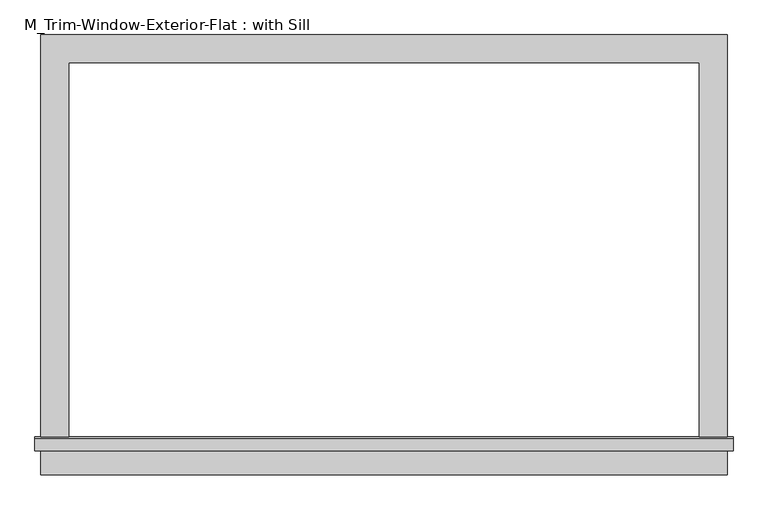
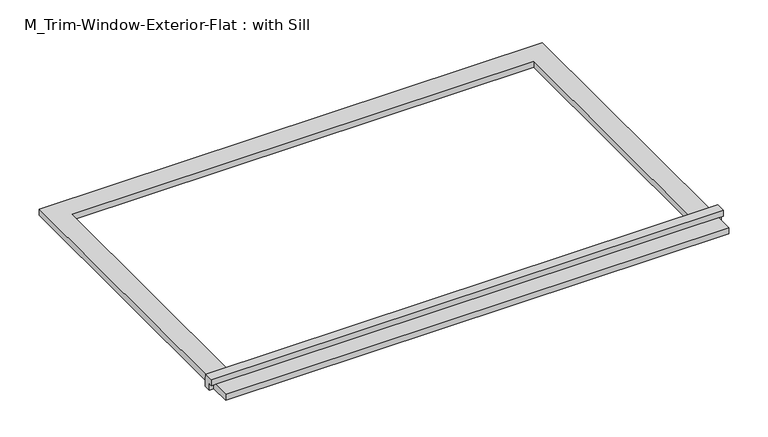
"""IFC4 building model written with IfcOpenShell, lengths in millimetres: proxy geometry, M_Trim-Window-Exterior-Flat : with Sill."""

from ifc_helpers import new_model, si_unit, frame, origin, origin_with_axes, place, context, project, spatial, polyline, outline, extrude, source, transform, mapped, element, save


def m_trim_window_exterior_flat_with_sill_2a9c44ae(model_context):
    return source(origin(), model_context, "Body", "SweptSolid", [
        extrude(outline(polyline([(733.1, -820.4323709), (733.1, -880.4323709), (-733.1, -880.4323709), (-733.1, -820.4323709), (733.1, -820.4323709)])), origin_with_axes(), (0.0, 0.0, 1.0), 19.05),
        extrude(outline(polyline([(-830.0, 38.1), (-802.4580645, 38.1), (-800.0, 19.05), (-800.0, 0.0), (-820.4323709, 0.0), (-820.4323709, 19.05), (-830.0, 19.05), (-830.0, 38.1)])), frame((-745.8, 0.0, 0.0), z_axis=(1.0, 0.0, 0.0), x_axis=(0.0, 1.0, 0.0)), (0.0, 0.0, 1.0), 1491.6),
        extrude(outline(polyline([(-733.1, 60.0), (733.1, 60.0), (733.1, -800.0), (673.1, -800.0), (673.1, 0.0), (-673.1, 0.0), (-673.1, -800.0), (-733.1, -800.0), (-733.1, 60.0)])), origin_with_axes(), (0.0, 0.0, 1.0), 19.05),
    ])


if __name__ == "__main__":
    model = new_model("IFC4")
    model_context = context("Model", 3, world=origin())
    ifc_project = project(units=[si_unit("LENGTHUNIT", "METRE", prefix="MILLI")], contexts=[model_context])
    site = spatial("IfcSite", under=ifc_project)
    building = spatial("IfcBuilding", under=site)
    placement = place(None, origin())
    m_trim_window_exterior_flat_with_sill_shape = m_trim_window_exterior_flat_with_sill_2a9c44ae(model_context)
    element("IfcBuildingElementProxy", 1, Name="M_Trim-Window-Exterior-Flat : with Sill", ObjectType="M_Trim-Window-Exterior-Flat : with Sill", at=placement, inside=building, context=model_context, shape_type="MappedRepresentation", body=[
        mapped(m_trim_window_exterior_flat_with_sill_shape, transform((0.0, 0.0, 0.0), x_axis=(1.0, 0.0, 0.0), y_axis=(0.0, 1.0, 0.0), z_axis=(0.0, 0.0, 1.0))),
    ])
    save(model, "model.ifc")

# Revit data of these elements
# Type "M_Trim-Window-Exterior-Flat : with Sill"
#   Trim Width = 0' - 2.3622"
#   Trim Thickness_Picture Frame = 0' - 1.1811"
#   Trim Thickness_with Sill = 0' - 0 3/4"
#   Sill Thickness = 0' - 1.1811"
#   Opening Width [instance default] = 1' - 11.62205"
#   Opening Height [instance default] = 2' - 11.43307"
#   Default Elevation = 3' - 11.24409"
#   Sill = yes
#   Picture Frame = no
#   Trim Material [instance default] = none
# Element 1 (IfcBuildingElementProxy, "M_Trim-Window-Exterior-Flat : with Sill")
#   Opening Width = 4' - 5"
#   Opening Height = 2' - 7.49606"
#   Trim Material = Clad - White
#   Materials on its faces: "Clad - White"
# Materials
#   "Clad - White": class "Wood", colour RGB 242 242 238, transparency 0, Cost = 0
